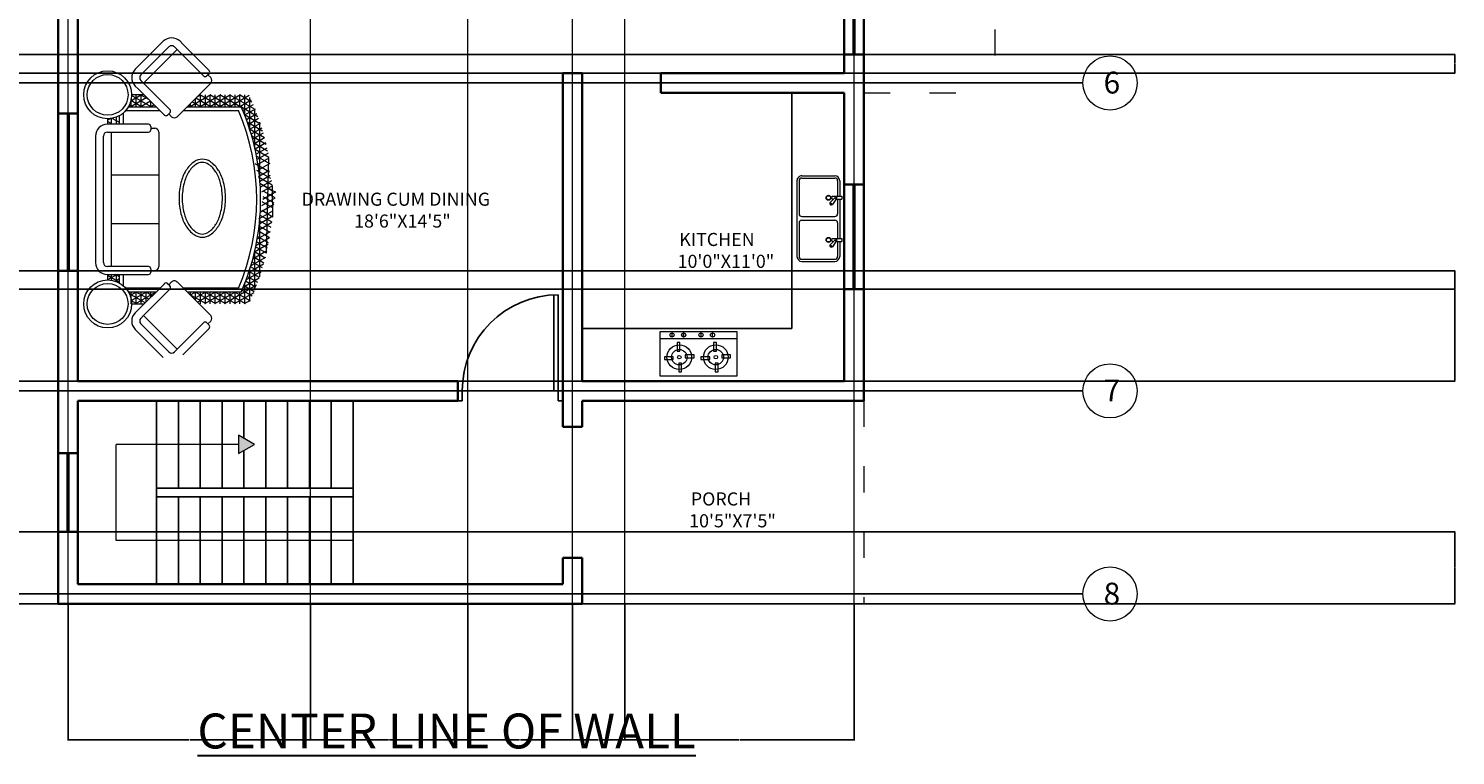
# Model space of a CAD drawing. Units: inches. Extents: x 5716 to 6907, y 12769 to 13594.
# Tile 11 of 17: x 6254 to 6907, y 12772 to 13105. Entities that reach past the tile are written whole.
import ezdxf

# ---------------------------------------------------------------- set-up
doc = ezdxf.new("R2010")
doc.units = ezdxf.units.IN
doc.linetypes.add('ACAD_ISO03W100', pattern=[30, 12, -18])
for name, color, linetype, lineweight in [('A-ANNO-DIMS', 2, 'Continuous', 18), ('A-ANNO-SYMB', 7, 'Continuous', 18), ('A-ANNO-TEXT', 7, 'Continuous', 30), ('A-AREA-IDEN', 7, 'Continuous', 18), ('A-DOOR', 4, 'Continuous', 25), ('A-EQPM', 8, 'Continuous', 18), ('A-FLOR-CASE', 7, 'Continuous', 25), ('A-FLOR-FIXT', 9, 'Continuous', 18), ('A-FLOR-OVHD', 8, 'ACAD_ISO03W100', 18), ('A-FLOR-STRS', 7, 'Continuous', 25), ('A-FURN', 8, 'Continuous', 18), ('A-GLAZ', 4, 'Continuous', 18), ('A-GRID', 8, 'Continuous', 13), ('A-GRID-IDEN', 7, 'Continuous', 18), ('A-WALL', 7, 'Continuous', 35)]:
    doc.layers.add(name, color=color, linetype=linetype, lineweight=lineweight)
doc.styles.get("Standard").update_dxf_attribs({"font": 'arial.ttf'})
doc.dimstyles.get("Standard").update_dxf_attribs({"dimtxt": 0.18, "dimasz": 0.18, "dimexe": 0.18, "dimexo": 0.0625, "dimgap": 0.09, "dimtad": 0, "dimtih": 1, "dimtoh": 1, "dimdec": 4, "dimzin": 0, "dimdsep": 46, "dimtxsty": 'Standard', "dimcen": 0.09, "dimadec": 0, "dimazin": 0, "dimtfac": 1, "dimtdec": 4, "dimtofl": 0, "dimtmove": 0, "dimatfit": 3, "dimfxl": 1, "dimtolj": 1, "dimtzin": 0, "dimarcsym": 0})

# ---------------------------------------------------------------- blocks, each defined once
blk = doc.blocks.new('A$C7A76439A')
for p, q in [((2799, 2282), (1199, 2282)), ((1199, 2182), (2799, 2182)), ((949, 1978), (1036, 2128)), ((959, 2017), (1049, 2017)), ((994, 1978), (964, 2030)), ((976, 2080), (1049, 2080)), ((1049, 2128), (980, 2128)), ((1049, 2008), (980, 2128)), ((1021, 1978), (1049, 2027)), ((1049, 2132), (1049, 2082)), ((1049, 2082), (1049, 1612)), ((1149, 1612), (1149, 2132)), ((2849, 2082), (1149, 2082)), ((1695, 2082), (1695, 1482)), ((2308, 2082), (2308, 1482)), ((2849, 2132), (2849, 1612)), ((2949, 2082), (2949, 2132)), ((3018, 2128), (2949, 2128)), ((2949, 2068), (2984, 2128)), ((2949, 1612), (2949, 2082)), ((2949, 2080), (3021, 2080)), ((2949, 2017), (3039, 2017)), ((2970, 1978), (3023, 2071)), ((3019, 2095), (3000, 2128)), ((3042, 1978), (3050, 1992)), ((677, 1830), (827, 1830)), ((677, 1758), (718, 1828)), ((677, 1825), (677, 1667)), ((690, 1655), (805, 1853)), ((827, 1642), (720, 1828)), ((827, 1767), (783, 1844)), ((827, 1517), (827, 1865)), ((877, 1467), (877, 1901)), ((905, 1928), (1049, 1928)), ((941, 1978), (1049, 1978)), ((2949, 1978), (3057, 1978)), ((2949, 1928), (3093, 1928)), ((3121, 1901), (3121, 1467)), ((3171, 1865), (3171, 1517)), ((3171, 1826), (3188, 1856)), ((3171, 1701), (3247, 1834)), ((3286, 1633), (3171, 1833)), ((3171, 1830), (3268, 1830)), ((3171, 1576), (3314, 1825)), ((3321, 1698), (3241, 1836)), ((3321, 1823), (3320, 1825)), ((3321, 1667), (3321, 1825)), ((354, 1779), (0, 1425)), ((71, 1354), (424, 1708)), ((106, 1248), (530, 1673)), ((530, 1673), (495, 1708)), ((863, 1340), (530, 1673)), ((601, 1743), (566, 1779)), ((933, 1411), (601, 1743)), ((827, 1517), (677, 1777)), ((677, 1767), (827, 1767)), ((677, 1705), (827, 1705)), ((702, 1642), (827, 1642)), ((736, 1609), (827, 1768)), ((781, 1563), (827, 1643)), ((3065, 1411), (3397, 1743)), ((3135, 1340), (3468, 1673)), ((3171, 1767), (3321, 1767)), ((3241, 1587), (3171, 1708)), ((3171, 1705), (3321, 1705)), ((3260, 1607), (3321, 1711)), ((3397, 1743), (3432, 1779)), ((3468, 1673), (3503, 1708)), ((3892, 1248), (3468, 1673)), ((3927, 1354), (3574, 1708)), ((3644, 1779), (3998, 1425)), ((765, 1580), (827, 1580)), ((1099, 1582), (1079, 1582)), ((1119, 1582), (1099, 1582)), ((1099, 1582), (1099, 1532)), ((2849, 1482), (1149, 1482)), ((2899, 1582), (2879, 1582)), ((2919, 1582), (2899, 1582)), ((2899, 1582), (2899, 1532)), ((3195, 1541), (3171, 1583)), ((3171, 1580), (3233, 1580)), ((3171, 1517), (3171, 1517)), ((106, 1248), (71, 1284)), ((905, 1340), (933, 1369)), ((919, 1354), (955, 1319)), ((3079, 1354), (3043, 1319)), ((3093, 1340), (3065, 1369)), ((3892, 1248), (3927, 1284)), ((368, 845), (35, 1178)), ((438, 916), (106, 1248)), ((530, 824), (955, 1248)), ((677, 883), (798, 1092)), ((827, 1017), (789, 1083)), ((827, 441), (827, 1121)), ((877, 474), (880, 1173)), ((3468, 824), (3043, 1248)), ((3121, 1171), (3121, 474)), ((3171, 1121), (3171, 441)), ((3171, 1076), (3187, 1105)), ((3321, 823), (3171, 1083)), ((3560, 916), (3892, 1248)), ((3630, 845), (3963, 1178)), ((3998, 1213), (3963, 1178)), ((677, 758), (827, 1018)), ((677, 955), (827, 955)), ((827, 767), (698, 991)), ((724, 1017), (827, 1017)), ((827, 892), (743, 1037)), ((786, 1080), (827, 1080)), ((3171, 1080), (3212, 1080)), ((3171, 951), (3233, 1059)), ((3171, 1017), (3274, 1017)), ((3171, 826), (3279, 1013)), ((3171, 701), (3321, 961)), ((3321, 698), (3171, 958)), ((3171, 955), (3321, 955)), ((3321, 948), (3290, 1002)), ((410, 845), (438, 874)), ((424, 859), (460, 824)), ((827, 642), (677, 902)), ((677, 633), (827, 893)), ((677, 892), (827, 892)), ((677, 830), (827, 830)), ((827, 517), (677, 777)), ((677, 508), (827, 768)), ((677, 767), (827, 767)), ((3171, 892), (3321, 892)), ((3171, 576), (3321, 836)), ((3321, 573), (3171, 833)), ((3171, 830), (3321, 830)), ((3171, 767), (3321, 767)), ((3574, 859), (3538, 824)), ((3588, 845), (3560, 874)), ((677, 705), (827, 705)), ((913, 244), (677, 652)), ((677, 383), (827, 643)), ((677, 642), (827, 642)), ((677, 580), (827, 580)), ((3134, 263), (3321, 586)), ((3171, 451), (3321, 711)), ((3321, 448), (3171, 708)), ((3171, 705), (3321, 705)), ((3171, 642), (3321, 642)), ((3311, 340), (3171, 583)), ((3171, 580), (3321, 580)), ((819, 281), (677, 527)), ((677, 517), (827, 517)), ((677, 455), (827, 455)), ((722, 324), (677, 402)), ((677, 392), (944, 392)), ((717, 326), (827, 518)), ((774, 300), (850, 431)), ((832, 276), (908, 407)), ((1004, 210), (886, 416)), ((891, 252), (966, 384)), ((950, 230), (1026, 362)), ((1093, 181), (979, 379)), ((2863, 169), (2975, 363)), ((2951, 196), (3067, 398)), ((3079, 241), (3003, 373)), ((3041, 227), (3163, 437)), ((3054, 392), (3321, 392)), ((3138, 264), (3062, 396)), ((3196, 289), (3121, 419)), ((3171, 517), (3321, 517)), ((3254, 314), (3171, 458)), ((3171, 455), (3321, 455)), ((3229, 303), (3321, 461)), ((709, 330), (1121, 330)), ((853, 267), (1349, 267)), ((1010, 209), (1086, 341)), ((1021, 205), (1744, 205)), ((1180, 156), (1070, 346)), ((1070, 188), (1147, 322)), ((1132, 170), (1209, 303)), ((1265, 133), (1159, 318)), ((1194, 152), (1271, 286)), ((1349, 114), (1245, 293)), ((1256, 135), (1334, 271)), ((1320, 120), (1398, 257)), ((1431, 97), (1330, 272)), ((1384, 106), (1463, 244)), ((1511, 83), (1412, 254)), ((1449, 94), (1528, 232)), ((1590, 71), (1494, 238)), ((1514, 82), (1595, 222)), ((1581, 72), (1662, 213)), ((1706, 50), (1607, 220)), ((1643, 60), (1723, 199)), ((1785, 38), (1688, 205)), ((1709, 49), (1790, 189)), ((1852, 43), (1749, 222)), ((1934, 26), (1833, 201)), ((2014, 12), (1916, 182)), ((2169, 45), (2089, 184)), ((2100, 34), (2198, 203)), ((2234, 57), (2155, 195)), ((2180, 47), (2280, 220)), ((2299, 71), (2220, 207)), ((2254, 205), (2977, 205)), ((2261, 63), (2363, 240)), ((2363, 85), (2284, 221)), ((2344, 81), (2449, 263)), ((2452, 77), (2371, 218)), ((2518, 88), (2438, 227)), ((2449, 77), (2547, 246)), ((2584, 100), (2504, 238)), ((2529, 90), (2629, 263)), ((2648, 113), (2569, 250)), ((2610, 105), (2712, 283)), ((2712, 128), (2633, 264)), ((2649, 267), (3145, 267)), ((2693, 124), (2798, 306)), ((2775, 144), (2697, 279)), ((2837, 161), (2760, 295)), ((2777, 145), (2885, 332)), ((2899, 179), (2822, 313)), ((2877, 330), (3289, 330)), ((2960, 199), (2883, 332)), ((3020, 220), (2943, 352)), ((1320, 120), (2529, 90)), ((1775, 39), (1857, 180)), ((1775, 39), (2169, 45)), ((1887, 35), (1966, 172)), ((1952, 23), (2032, 161)), ((2093, 0), (1997, 167)), ((2018, 11), (2098, 151)), ((2084, 1), (2165, 142))]:
    blk.add_line(p, q)
for centre, radius in [((677, 2128), 303), ((677, 2128), 258), ((3321, 2128), 303), ((3321, 2128), 258)]:
    blk.add_circle(centre, radius)
for centre, radius, start, end in [((1199, 2132), 150, 90, 180), ((1199, 2132), 50, 90, 180), ((2799, 2132), 150, 0, 90), ((2799, 2132), 50, 0, 90), ((460, 1673), 150, 45, 135), ((3538, 1673), 150, 45, 135), ((460, 1673), 50, 45, 135), ((3538, 1673), 50, 45, 135), ((1079, 1612), 30, 180, 270), ((1149, 1532), 50, 180, 270), ((1119, 1612), 30, 270, 0), ((2879, 1612), 30, 180, 270), ((2849, 1532), 50, 270, 0), ((2919, 1612), 30, 270, 0), ((106, 1319), 50, 135, 225), ((884, 1362), 30, 225, 315), ((912, 1390), 30, 315, 45), ((919, 1284), 50, 315, 45), ((3079, 1284), 50, 135, 225), ((3086, 1390), 30, 135, 225), ((3114, 1362), 30, 225, 315), ((3892, 1319), 50, 315, 45), ((3892, 1319), 150, 315, 45), ((1851, 828), 362, 120.7882, 145.1939), ((1851, 828), 322, 120.7882, 145.1939), ((1949, 662), 555, 103.8638, 120.7882), ((1949, 662), 515, 103.8638, 120.7882), ((2014, 400), 825, 90, 103.8638), ((2014, 400), 785, 90, 103.8638), ((2014, 400), 825, 76.1362, 90), ((2014, 400), 785, 76.1362, 90), ((2079, 662), 515, 59.2118, 76.1362), ((2079, 662), 555, 59.2118, 76.1362), ((2177, 828), 322, 34.8061, 59.2118), ((2177, 828), 362, 34.8061, 59.2118), ((417, 895), 30, 315, 45), ((1702, 931), 181, 145.1939, 180), ((1702, 931), 181, 180, 214.8061), ((1702, 931), 141, 145.1939, 180), ((1702, 931), 141, 180, 214.8061), ((2326, 931), 141, 0, 34.8061), ((2326, 931), 141, 325.1939, 0), ((2326, 931), 181, 0, 34.8061), ((2326, 931), 181, 325.1939, 0), ((3581, 895), 30, 135, 225), ((389, 867), 30, 225, 315), ((495, 859), 50, 225, 315), ((1851, 1035), 362, 214.8061, 239.2118), ((1851, 1035), 322, 214.8061, 239.2118), ((1949, 1200), 555, 239.2118, 256.1362), ((1949, 1200), 515, 239.2118, 256.1362), ((2079, 1200), 515, 283.8638, 300.7882), ((2079, 1200), 555, 283.8638, 300.7882), ((2177, 1035), 322, 300.7882, 325.1939), ((2177, 1035), 362, 300.7882, 325.1939), ((3503, 859), 50, 225, 315), ((3609, 867), 30, 225, 315), ((2014, 1462), 825, 256.1362, 270), ((2014, 1462), 785, 256.1362, 270), ((2014, 1462), 785, 270, 283.8638), ((2014, 1462), 825, 270, 283.8638), ((1999, 3092), 2899, 246.1589, 293.8411), ((1999, 3092), 2849, 246.8124, 293.1876)]:
    blk.add_arc(centre, radius, start, end)
blk = doc.blocks.new('A$C233D5AEA')
at = {"ltscale": 1000}
for p, q in [((20, 613), (20, 755)), ((40, 613), (40, 755)), ((375, 800), (65, 800)), ((375, 780), (65, 780)), ((400, 440), (400, 755)), ((420, 45), (420, 755)), ((55, 613), (0, 613)), ((0, 586), (0, 613)), ((89, 586), (0, 586)), ((20, 218), (20, 586)), ((40, 440), (40, 586)), ((51, 606), (87, 664)), ((112, 647), (63, 598)), ((88, 613), (78, 613)), ((87, 664), (112, 647)), ((375, 415), (65, 415)), ((40, 218), (40, 355)), ((51, 211), (87, 268)), ((375, 380), (65, 380)), ((87, 268), (112, 252)), ((400, 45), (400, 355)), ((55, 218), (0, 218)), ((0, 191), (0, 218)), ((89, 191), (0, 191)), ((20, 45), (20, 191)), ((40, 45), (40, 191)), ((112, 252), (63, 202)), ((88, 218), (78, 218)), ((375, 20), (65, 20)), ((375, 0), (65, 0))]:
    blk.add_line(p, q, dxfattribs=at)
for centre, radius in [((55, 600), 7.79), ((125, 599), 23.1), ((125, 599), 19.5), ((55, 204), 7.79), ((125, 205), 23.1), ((125, 205), 19.5)]:
    blk.add_circle(centre, radius, dxfattribs=at)
for centre, radius, start, end in [((65, 755), 45, 90, 180), ((65, 755), 25, 90, 180), ((375, 755), 45, 0, 90), ((375, 755), 25, 0, 90), ((98, 652), 15.3, 340.4622, 131.655), ((82, 599), 14.9, 296.6237, 67.0796), ((65, 440), 25, 180, 270), ((375, 440), 25, 270, 0), ((65, 355), 25, 90, 180), ((98, 257), 15.3, 340.4691, 131.6481), ((375, 355), 25, 0, 90), ((82, 204), 14.9, 296.6237, 67.0796), ((65, 45), 45, 180, 270), ((65, 45), 25, 180, 270), ((375, 45), 45, 270, 0), ((375, 45), 25, 270, 0)]:
    blk.add_arc(centre, radius, start, end, dxfattribs=at)
blk = doc.blocks.new('A$C3BE07067')
at = {"rotation": 270}
blk.add_blockref('A$C233D5AEA', (0, 420), dxfattribs=at)
blk = doc.blocks.new('A$C67D72025')
at = {"ltscale": 1000}
for p, q in [((386, 234), (386, 209)), ((465, 234), (386, 234)), ((386, 209), (465, 209)), ((465, 209), (465, 234)), ((694, 60), (0, 60))]:
    blk.add_line(p, q, dxfattribs=at)
for points in [[(694, 397), (0, 397), (0, 0), (694, 0)], [(196, 284), (196, 362), (171, 362), (171, 284)], [(523, 284), (523, 362), (499, 362), (499, 284)], [(137, 234), (58, 234), (58, 209), (137, 209)], [(186, 175), (186, 96), (211, 96), (211, 175)], [(245, 225), (324, 225), (324, 250), (245, 250)], [(514, 175), (514, 96), (539, 96), (539, 175)], [(573, 225), (652, 225), (652, 250), (573, 250)], [(223, 47), (220, 47), (220, 10), (223, 10)], [(326, 47), (322, 47), (322, 10), (326, 10)], [(483, 47), (479, 47), (479, 10), (483, 10)], [(585, 47), (582, 47), (582, 10), (585, 10)]]:
    blk.add_lwpolyline(points, close=True, dxfattribs=at)
for centre, radius in [((191, 229), 111), ((191, 229), 69.6), ((519, 229), 111), ((519, 229), 69.6), ((191, 229), 15.5), ((519, 229), 15.5), ((220, 29), 18.6), ((324, 29), 18.6), ((480, 29), 18.6), ((584, 29), 18.6)]:
    blk.add_circle(centre, radius, dxfattribs=at)
blk = doc.blocks.new('DOOR-SWING-48IN')
for p, q in [((-2, 43.95), (-2, 0)), ((0, 44), (0, 0)), ((-46, 0), (-44, 0)), ((-44, -4.5), (-46, -4.5)), ((-44, 0), (-44, -4.5)), ((0, 0), (-2, 0)), ((2, 0), (0, 0)), ((0, 0), (0, -4.5)), ((0, -4.5), (2, -4.5))]:
    blk.add_line(p, q)
blk.add_arc((0, 0), 44, 90, 180)
blk = doc.blocks.new('WIN-GLAZING-72IN')
for p, q in [((0, 0), (0, -72)), ((1, 0), (1, -72))]:
    blk.add_line(p, q)
blk = doc.blocks.new('WIN-GLAZING-48IN')
for p, q in [((0, 0), (0, 48)), ((1, 0), (1, 48))]:
    blk.add_line(p, q)
blk = doc.blocks.new('WIN-GLAZING-36IN')
for p, q in [((0, 0), (0, 36)), ((1, 0), (1, 36))]:
    blk.add_line(p, q)
blk = doc.blocks.new('STAIR-RETURN-FLIGHT')
for p, q in [((0, 84), (0, 44)), ((10, 84), (10, 44)), ((20, 84), (20, 44)), ((30, 84), (30, 44)), ((40, 84), (40, 66.79)), ((50, 84), (50, 44)), ((60, 84), (60, 44)), ((70, 84), (70, 44)), ((80, 84), (80, 44)), ((90, 84), (90, 44)), ((40, 61.21), (40, 44)), ((0, 44), (90, 44)), ((0, 40), (0, 44)), ((0, 40), (90, 40)), ((0, 40), (0, 0)), ((10, 40), (10, 0)), ((20, 40), (20, 0)), ((30, 40), (30, 0)), ((40, 40), (40, 0)), ((50, 40), (50, 0)), ((60, 40), (60, 0)), ((70, 40), (70, 0)), ((80, 40), (80, 0)), ((90, 40), (90, 44)), ((90, 40), (90, 0))]:
    blk.add_line(p, q)
blk = doc.blocks.new('COUNTER-L-KITCHEN')
for p in [(0, 108), (-96, 0)]:
    blk.add_line(p, (0, 0))
blk = doc.blocks.new('*D52')
at = {"layer": 'A-ANNO-DIMS', "color": 0, "lineweight": -2, "transparency": 16777216}
for p, q in [((6267.34, 13440.15), (5716.04, 13440.15)), ((5716.22, 13439.97), (5716.22, 13140.83)), ((5716.22, 12841.33), (5716.22, 13140.47)), ((6267.34, 12841.15), (5716.04, 12841.15))]:
    blk.add_line(p, q, dxfattribs=at)
at = {"layer": 'A-ANNO-DIMS', "color": 0, "transparency": 16777216}
for points in [[(5716.19, 13439.97), (5716.25, 13439.97), (5716.22, 13440.15)], [(5716.19, 12841.33), (5716.25, 12841.33), (5716.22, 12841.15)]]:
    blk.add_solid(points, dxfattribs=at)
at = {"layer": 'Defpoints', "color": 0, "transparency": 16777216}
for p in [(6267.41, 13440.15), (5716.22, 12841.15), (6267.41, 12841.15)]:
    blk.add_point(p, dxfattribs=at)
at = {"layer": 'A-ANNO-DIMS', "color": 0, "transparency": 16777216, "insert": (5716.22, 13140.65), "char_height": 0.18, "attachment_point": 5}
blk.add_mtext('\\A1;599', dxfattribs=at)
blk = doc.blocks.new('*D53')
at = {"layer": 'A-ANNO-DIMS', "color": 0, "lineweight": -2, "transparency": 16777216}
for p, q in [((6271.91, 12841.09), (6271.91, 12778.62)), ((6382.91, 12841.09), (6382.91, 12778.62)), ((6272.09, 12778.8), (6327.14, 12778.8)), ((6382.73, 12778.8), (6327.67, 12778.8))]:
    blk.add_line(p, q, dxfattribs=at)
at = {"layer": 'A-ANNO-DIMS', "color": 0, "transparency": 16777216}
for points in [[(6272.09, 12778.83), (6272.09, 12778.77), (6271.91, 12778.8)], [(6382.73, 12778.83), (6382.73, 12778.77), (6382.91, 12778.8)]]:
    blk.add_solid(points, dxfattribs=at)
at = {"layer": 'Defpoints', "color": 0, "transparency": 16777216}
for p in [(6271.91, 12841.15), (6382.91, 12841.15), (6382.91, 12778.8)]:
    blk.add_point(p, dxfattribs=at)
at = {"layer": 'A-ANNO-DIMS', "color": 0, "transparency": 16777216, "insert": (6327.41, 12778.8), "char_height": 0.18, "attachment_point": 5}
blk.add_mtext('\\A1;111', dxfattribs=at)
blk = doc.blocks.new('*D54')
at = {"layer": 'A-ANNO-DIMS', "color": 0, "lineweight": -2, "transparency": 16777216}
for p, q in [((6382.91, 12841.09), (6382.91, 12778.62)), ((6454.91, 12841.09), (6454.91, 12778.62)), ((6383.09, 12778.8), (6418.69, 12778.8)), ((6454.73, 12778.8), (6419.12, 12778.8))]:
    blk.add_line(p, q, dxfattribs=at)
at = {"layer": 'A-ANNO-DIMS', "color": 0, "transparency": 16777216}
for points in [[(6383.09, 12778.83), (6383.09, 12778.77), (6382.91, 12778.8)], [(6454.73, 12778.83), (6454.73, 12778.77), (6454.91, 12778.8)]]:
    blk.add_solid(points, dxfattribs=at)
at = {"layer": 'Defpoints', "color": 0, "transparency": 16777216}
for p in [(6382.91, 12841.15), (6454.91, 12841.15), (6454.91, 12778.8)]:
    blk.add_point(p, dxfattribs=at)
at = {"layer": 'A-ANNO-DIMS', "color": 0, "transparency": 16777216, "insert": (6418.91, 12778.8), "char_height": 0.18, "attachment_point": 5}
blk.add_mtext('\\A1;72', dxfattribs=at)
blk = doc.blocks.new('*D55')
at = {"layer": 'A-ANNO-DIMS', "color": 0, "lineweight": -2, "transparency": 16777216}
for p, q in [((6454.91, 12841.09), (6454.91, 12778.62)), ((6502.91, 12841.09), (6502.91, 12778.62)), ((6455.09, 12778.8), (6478.68, 12778.8)), ((6502.73, 12778.8), (6479.13, 12778.8))]:
    blk.add_line(p, q, dxfattribs=at)
at = {"layer": 'A-ANNO-DIMS', "color": 0, "transparency": 16777216}
for points in [[(6455.09, 12778.83), (6455.09, 12778.77), (6454.91, 12778.8)], [(6502.73, 12778.83), (6502.73, 12778.77), (6502.91, 12778.8)]]:
    blk.add_solid(points, dxfattribs=at)
at = {"layer": 'Defpoints', "color": 0, "transparency": 16777216}
for p in [(6454.91, 12841.15), (6502.91, 12841.15), (6502.91, 12778.8)]:
    blk.add_point(p, dxfattribs=at)
at = {"layer": 'A-ANNO-DIMS', "color": 0, "transparency": 16777216, "insert": (6478.91, 12778.8), "char_height": 0.18, "attachment_point": 5}
blk.add_mtext('\\A1;48', dxfattribs=at)
blk = doc.blocks.new('*D56')
at = {"layer": 'A-ANNO-DIMS', "color": 0, "lineweight": -2, "transparency": 16777216}
for p, q in [((6502.91, 12841.09), (6502.91, 12778.62)), ((6526.91, 12841.09), (6526.91, 12778.62)), ((6503.09, 12778.8), (6514.69, 12778.8)), ((6526.73, 12778.8), (6515.13, 12778.8))]:
    blk.add_line(p, q, dxfattribs=at)
at = {"layer": 'A-ANNO-DIMS', "color": 0, "transparency": 16777216}
for points in [[(6503.09, 12778.83), (6503.09, 12778.77), (6502.91, 12778.8)], [(6526.73, 12778.83), (6526.73, 12778.77), (6526.91, 12778.8)]]:
    blk.add_solid(points, dxfattribs=at)
at = {"layer": 'Defpoints', "color": 0, "transparency": 16777216}
for p in [(6502.91, 12841.15), (6526.91, 12841.15), (6526.91, 12778.8)]:
    blk.add_point(p, dxfattribs=at)
at = {"layer": 'A-ANNO-DIMS', "color": 0, "transparency": 16777216, "insert": (6514.91, 12778.8), "char_height": 0.18, "attachment_point": 5}
blk.add_mtext('\\A1;24', dxfattribs=at)
blk = doc.blocks.new('*D57')
at = {"layer": 'A-ANNO-DIMS', "color": 0, "lineweight": -2, "transparency": 16777216}
for p, q in [((6526.91, 12841.09), (6526.91, 12778.62)), ((6631.91, 12841.09), (6631.91, 12778.62)), ((6527.09, 12778.8), (6579.13, 12778.8)), ((6631.73, 12778.8), (6579.69, 12778.8))]:
    blk.add_line(p, q, dxfattribs=at)
at = {"layer": 'A-ANNO-DIMS', "color": 0, "transparency": 16777216}
for points in [[(6527.09, 12778.83), (6527.09, 12778.77), (6526.91, 12778.8)], [(6631.73, 12778.83), (6631.73, 12778.77), (6631.91, 12778.8)]]:
    blk.add_solid(points, dxfattribs=at)
at = {"layer": 'Defpoints', "color": 0, "transparency": 16777216}
for p in [(6526.91, 12841.15), (6631.91, 12841.15), (6631.91, 12778.8)]:
    blk.add_point(p, dxfattribs=at)
at = {"layer": 'A-ANNO-DIMS', "color": 0, "transparency": 16777216, "insert": (6579.41, 12778.8), "char_height": 0.18, "attachment_point": 5}
blk.add_mtext('\\A1;105', dxfattribs=at)
blk = doc.blocks.new('*D62')
at = {"layer": 'A-ANNO-DIMS', "color": 0, "lineweight": -2, "transparency": 16777216}
for p, q in [((6736.67, 13120.65), (5716.04, 13120.65)), ((5716.22, 13120.47), (5716.22, 13100.33)), ((5716.22, 13079.83), (5716.22, 13099.97)), ((6736.67, 13079.65), (5716.04, 13079.65))]:
    blk.add_line(p, q, dxfattribs=at)
at = {"layer": 'A-ANNO-DIMS', "color": 0, "transparency": 16777216}
for points in [[(5716.19, 13120.47), (5716.25, 13120.47), (5716.22, 13120.65)], [(5716.19, 13079.83), (5716.25, 13079.83), (5716.22, 13079.65)]]:
    blk.add_solid(points, dxfattribs=at)
at = {"layer": 'Defpoints', "color": 0, "transparency": 16777216}
for p in [(6736.73, 13120.65), (5716.22, 13079.65), (6736.73, 13079.65)]:
    blk.add_point(p, dxfattribs=at)
at = {"layer": 'A-ANNO-DIMS', "color": 0, "transparency": 16777216, "insert": (5716.22, 13100.15), "char_height": 0.18, "attachment_point": 5}
blk.add_mtext('\\A1;41', dxfattribs=at)
blk = doc.blocks.new('*D63')
at = {"layer": 'A-ANNO-DIMS', "color": 0, "lineweight": -2, "transparency": 16777216}
for p, q in [((6736.67, 13079.65), (5716.04, 13079.65)), ((5716.22, 13079.47), (5716.22, 13009.33)), ((5716.22, 12938.83), (5716.22, 13008.97)), ((6736.67, 12938.65), (5716.04, 12938.65))]:
    blk.add_line(p, q, dxfattribs=at)
at = {"layer": 'A-ANNO-DIMS', "color": 0, "transparency": 16777216}
for points in [[(5716.19, 13079.47), (5716.25, 13079.47), (5716.22, 13079.65)], [(5716.19, 12938.83), (5716.25, 12938.83), (5716.22, 12938.65)]]:
    blk.add_solid(points, dxfattribs=at)
at = {"layer": 'Defpoints', "color": 0, "transparency": 16777216}
for p in [(6736.73, 13079.65), (5716.22, 12938.65), (6736.73, 12938.65)]:
    blk.add_point(p, dxfattribs=at)
at = {"layer": 'A-ANNO-DIMS', "color": 0, "transparency": 16777216, "insert": (5716.22, 13009.15), "char_height": 0.18, "attachment_point": 5}
blk.add_mtext('\\A1;141', dxfattribs=at)
blk = doc.blocks.new('*D64')
at = {"layer": 'A-ANNO-DIMS', "color": 0, "lineweight": -2, "transparency": 16777216}
for p, q in [((6736.67, 12938.65), (5716.04, 12938.65)), ((5716.22, 12938.47), (5716.22, 12892.33)), ((5716.22, 12845.83), (5716.22, 12891.97)), ((6736.67, 12845.65), (5716.04, 12845.65))]:
    blk.add_line(p, q, dxfattribs=at)
at = {"layer": 'A-ANNO-DIMS', "color": 0, "transparency": 16777216}
for points in [[(5716.19, 12938.47), (5716.25, 12938.47), (5716.22, 12938.65)], [(5716.19, 12845.83), (5716.25, 12845.83), (5716.22, 12845.65)]]:
    blk.add_solid(points, dxfattribs=at)
at = {"layer": 'Defpoints', "color": 0, "transparency": 16777216}
for p in [(6736.73, 12938.65), (5716.22, 12845.65), (6736.73, 12845.65)]:
    blk.add_point(p, dxfattribs=at)
at = {"layer": 'A-ANNO-DIMS', "color": 0, "transparency": 16777216, "insert": (5716.22, 12892.15), "char_height": 0.18, "attachment_point": 5}
blk.add_mtext('\\A1;93', dxfattribs=at)
blk = doc.blocks.new('*D67')
at = {"layer": 'A-ANNO-DIMS', "color": 0, "lineweight": -2, "transparency": 16777216}
for p, q in [((5819.09, 12874.15), (6907.26, 12874.15)), ((6907.08, 12873.97), (6907.08, 12857.83)), ((6907.08, 12841.33), (6907.08, 12857.47)), ((5819.09, 12841.15), (6907.26, 12841.15))]:
    blk.add_line(p, q, dxfattribs=at)
at = {"layer": 'A-ANNO-DIMS', "color": 0, "transparency": 16777216}
for points in [[(6907.05, 12873.97), (6907.11, 12873.97), (6907.08, 12874.15)], [(6907.05, 12841.33), (6907.11, 12841.33), (6907.08, 12841.15)]]:
    blk.add_solid(points, dxfattribs=at)
at = {"layer": 'Defpoints', "color": 0, "transparency": 16777216}
for p in [(5819.02, 12874.15), (6907.08, 12874.15), (5819.02, 12841.15)]:
    blk.add_point(p, dxfattribs=at)
at = {"layer": 'A-ANNO-DIMS', "color": 0, "transparency": 16777216, "insert": (6907.08, 12857.65), "char_height": 0.18, "attachment_point": 5}
blk.add_mtext('\\A1;33', dxfattribs=at)
blk = doc.blocks.new('*D68')
at = {"layer": 'A-ANNO-DIMS', "color": 0, "lineweight": -2, "transparency": 16777216}
for p, q in [((5828.09, 12993.65), (6907.26, 12993.65)), ((6907.08, 12993.47), (6907.08, 12968.58)), ((6907.08, 12943.33), (6907.08, 12968.22)), ((5828.09, 12943.15), (6907.26, 12943.15))]:
    blk.add_line(p, q, dxfattribs=at)
at = {"layer": 'A-ANNO-DIMS', "color": 0, "transparency": 16777216}
for points in [[(6907.05, 12993.47), (6907.11, 12993.47), (6907.08, 12993.65)], [(6907.05, 12943.33), (6907.11, 12943.33), (6907.08, 12943.15)]]:
    blk.add_solid(points, dxfattribs=at)
at = {"layer": 'Defpoints', "color": 0, "transparency": 16777216}
for p in [(5828.02, 12993.65), (6907.08, 12993.65), (5828.02, 12943.15)]:
    blk.add_point(p, dxfattribs=at)
at = {"layer": 'A-ANNO-DIMS', "color": 0, "transparency": 16777216, "insert": (6907.08, 12968.4), "char_height": 0.18, "attachment_point": 5}
blk.add_mtext('\\A1;50.5', dxfattribs=at)
blk = doc.blocks.new('*D72')
at = {"layer": 'A-ANNO-DIMS', "color": 0, "lineweight": -2, "transparency": 16777216}
for p, q in [((6188.09, 12985.15), (6907.26, 12985.15)), ((6907.08, 12984.97), (6907.08, 12964.33)), ((6907.08, 12943.33), (6907.08, 12963.97)), ((6179.09, 12943.15), (6907.26, 12943.15))]:
    blk.add_line(p, q, dxfattribs=at)
at = {"layer": 'A-ANNO-DIMS', "color": 0, "transparency": 16777216}
for points in [[(6907.05, 12984.97), (6907.11, 12984.97), (6907.08, 12985.15)], [(6907.05, 12943.33), (6907.11, 12943.33), (6907.08, 12943.15)]]:
    blk.add_solid(points, dxfattribs=at)
at = {"layer": 'Defpoints', "color": 0, "transparency": 16777216}
for p in [(6188.02, 12985.15), (6907.08, 12985.15), (6179.02, 12943.15)]:
    blk.add_point(p, dxfattribs=at)
at = {"layer": 'A-ANNO-DIMS', "color": 0, "transparency": 16777216, "insert": (6907.08, 12964.15), "char_height": 0.18, "attachment_point": 5}
blk.add_mtext('\\A1;42', dxfattribs=at)
blk = doc.blocks.new('*D73')
at = {"layer": 'A-ANNO-DIMS', "color": 0, "lineweight": -2, "transparency": 16777216}
for p, q in [((6188.09, 13092.65), (6907.26, 13092.65)), ((6907.08, 13092.47), (6907.08, 13088.58)), ((6907.08, 13084.33), (6907.08, 13088.22)), ((6179.09, 13084.15), (6907.26, 13084.15))]:
    blk.add_line(p, q, dxfattribs=at)
at = {"layer": 'A-ANNO-DIMS', "color": 0, "transparency": 16777216}
for points in [[(6907.05, 13092.47), (6907.11, 13092.47), (6907.08, 13092.65)], [(6907.05, 13084.33), (6907.11, 13084.33), (6907.08, 13084.15)]]:
    blk.add_solid(points, dxfattribs=at)
at = {"layer": 'Defpoints', "color": 0, "transparency": 16777216}
for p in [(6188.02, 13092.65), (6907.08, 13092.65), (6179.02, 13084.15)]:
    blk.add_point(p, dxfattribs=at)
at = {"layer": 'A-ANNO-DIMS', "color": 0, "transparency": 16777216, "insert": (6907.08, 13088.4), "char_height": 0.18, "attachment_point": 5}
blk.add_mtext('\\A1;8.5', dxfattribs=at)

msp = doc.modelspace()

# ---------------------------------------------------------------- hatches: boundary and pattern name
at = {"layer": 'A-ANNO-SYMB'}
h = msp.add_hatch(color=256, dxfattribs=at)
h.dxf.hatch_style = 1
h.paths.add_polyline_path([(6357.24, 12914.15), (6349.99, 12918.34), (6349.99, 12909.96)])

# ---------------------------------------------------------------- linework, layer by layer
for p, q in [((6293.86, 12870.15), (6293.86, 12914.15)), ((6349.99, 12914.15), (6293.86, 12914.15)), ((6402.41, 12870.15), (6293.86, 12870.15))]:
    msp.add_line(p, q, dxfattribs=at)
msp.add_lwpolyline([(6357.24, 12914.15), (6349.99, 12918.34), (6349.99, 12909.96)], close=True, dxfattribs=at)
at = {"layer": 'A-FLOR-OVHD'}
for p, q in [((6696.41, 13194.15), (6696.41, 13075.15)), ((6636.41, 13075.15), (6696.41, 13075.15)), ((6636.41, 12934.15), (6636.41, 12841.15)), ((6507.41, 12841.15), (6636.41, 12841.15))]:
    msp.add_line(p, q, dxfattribs=at)
at = {"layer": 'A-GRID'}
for p, q in [((6271.91, 12841.15), (6271.91, 13514.96)), ((6382.91, 12841.15), (6382.91, 13514.96)), ((6454.91, 12841.15), (6454.91, 13514.96)), ((6502.91, 12841.15), (6502.91, 13514.96)), ((6526.91, 12841.15), (6526.91, 13514.96)), ((6631.91, 12841.15), (6631.91, 13514.96)), ((6267.41, 13079.65), (6736.73, 13079.65)), ((6267.41, 12938.65), (6736.73, 12938.65)), ((6267.41, 12845.65), (6736.73, 12845.65))]:
    msp.add_line(p, q, dxfattribs=at)
at = {"layer": 'A-GRID-IDEN'}
for centre in [(6749.12, 13079.65), (6749.12, 12938.65), (6749.12, 12845.65)]:
    msp.add_circle(centre, 12.4, dxfattribs=at)
at = {"layer": 'A-WALL'}
for p, q in [((6267.41, 13440.15), (6267.41, 12841.15)), ((6627.41, 13149.15), (6627.41, 13084.15)), ((6636.41, 13149.15), (6636.41, 12934.15)), ((6276.41, 13116.15), (6276.41, 12943.15)), ((6627.41, 13092.65), (6636.41, 13092.65)), ((6498.41, 13084.15), (6498.41, 12922.15)), ((6498.41, 13084.15), (6507.41, 13084.15)), ((6507.41, 13084.15), (6507.41, 12943.15)), ((6543.41, 13084.15), (6543.41, 13075.15)), ((6543.41, 13084.15), (6627.41, 13084.15)), ((6543.41, 13075.15), (6627.41, 13075.15)), ((6627.41, 13075.15), (6627.41, 12943.15)), ((6276.41, 13065.65), (6267.41, 13065.65)), ((6627.41, 13033.15), (6636.41, 13033.15)), ((6276.41, 12993.65), (6267.41, 12993.65)), ((6627.41, 12985.15), (6636.41, 12985.15)), ((6276.41, 12943.15), (6450.41, 12943.15)), ((6450.41, 12943.15), (6450.41, 12934.15)), ((6507.41, 12943.15), (6627.41, 12943.15)), ((6276.41, 12934.15), (6276.41, 12850.15)), ((6276.41, 12934.15), (6450.41, 12934.15)), ((6507.41, 12934.15), (6507.41, 12922.15)), ((6507.41, 12934.15), (6636.41, 12934.15)), ((6498.41, 12922.15), (6507.41, 12922.15)), ((6276.41, 12910.15), (6267.41, 12910.15)), ((6276.41, 12874.15), (6267.41, 12874.15)), ((6498.41, 12862.15), (6498.41, 12850.15)), ((6498.41, 12862.15), (6507.41, 12862.15)), ((6507.41, 12862.15), (6507.41, 12841.15)), ((6276.41, 12850.15), (6498.41, 12850.15)), ((6267.41, 12841.15), (6507.41, 12841.15))]:
    msp.add_line(p, q, dxfattribs=at)

# ---------------------------------------------------------------- block references
at = {"layer": 'A-DOOR'}
msp.add_blockref('DOOR-SWING-48IN', (6496.41, 12938.65), dxfattribs=at)
at = {"layer": 'A-EQPM', "xscale": 0.0509457092912183, "yscale": 0.0509457092912183, "zscale": 0.0509457092912183, "rotation": 180}
msp.add_blockref('A$C67D72025', (6578.27, 12965.75), dxfattribs=at)
at = {"layer": 'A-FLOR-CASE'}
msp.add_blockref('COUNTER-L-KITCHEN', (6603.41, 12967.15), dxfattribs=at)
at = {"layer": 'A-FLOR-FIXT', "xscale": 0.0489344977334652, "yscale": 0.0489344977334652, "zscale": 0.0489344977334652, "rotation": 270}
msp.add_blockref('A$C3BE07067', (6605.72, 13037.09), dxfattribs=at)
at = {"layer": 'A-FLOR-STRS'}
msp.add_blockref('STAIR-RETURN-FLIGHT', (6312.41, 12850.15), dxfattribs=at)
at = {"layer": 'A-FURN', "xscale": 0.0362164969968974, "yscale": 0.0362164969968974, "zscale": 0.0362164969968974, "rotation": 90}
msp.add_blockref('A$C7A76439A', (6367.07, 12953.94), dxfattribs=at)
at = {"layer": 'A-GLAZ'}
for name, p in [('WIN-GLAZING-48IN', (6631.41, 13092.65)), ('WIN-GLAZING-72IN', (6271.41, 13065.65)), ('WIN-GLAZING-48IN', (6631.41, 12985.15)), ('WIN-GLAZING-36IN', (6271.41, 12874.15))]:
    msp.add_blockref(name, p, dxfattribs=at)

# ---------------------------------------------------------------- texts
at = {"layer": 'A-ANNO-TEXT', "insert": (6331.1, 12790.92), "char_height": 16, "attachment_point": 1}
msp.add_mtext_dynamic_manual_height_columns('{\\LCENTER LINE OF WALL}', width=852.8728, gutter_width=12.5, heights=[0], dxfattribs=at)
at = {"layer": 'A-AREA-IDEN', "attachment_point": 1}
for s, width, heights, insert, char_height in [('DRAWING CUM DINING\\P^I18\'6"X14\'5"', 158.347, [0], (6378.87, 13029.41), 6), (' {\\H2.4x;KITCHEN\\P10\'0"X11\'0"}', 81.2135, [0], (6551.05, 13010.98), 2.5), (' {\\H2.4x;PORCH\\P10\'5"X7\'5"}', 95.0073, [19.73], (6556.34, 12892.17), 2.5)]:
    msp.add_mtext_dynamic_manual_height_columns(s, width=width, gutter_width=12.5, heights=heights, dxfattribs=dict(at, insert=insert, char_height=char_height))
at = {"layer": 'A-GRID-IDEN', "char_height": 10, "attachment_point": 1}
for s, insert in [('6', (6746.18, 13084.81)), ('7', (6746.18, 12943.81)), ('8', (6746.18, 12850.81))]:
    msp.add_mtext_dynamic_manual_height_columns(s, width=121.9272, gutter_width=12.5, heights=[0], dxfattribs=dict(at, insert=insert))

# ---------------------------------------------------------------- dimensions: what is measured, and where the dimension line sits
at = {"layer": 'A-ANNO-DIMS'}
for base, p1, p2, override, picture, middle in [((5716.22, 12841.15), (6267.41, 13440.15), (6267.41, 12841.15), {"dimdec": 0, "dimlfac": 1, "dimrnd": 0, "dimzin": 0, "dimdsep": 46, "dimlunit": 2}, '*D52', (5716.22, 13140.65)), ((5716.22, 13079.65), (6736.73, 13120.65), (6736.73, 13079.65), {"dimdec": 0, "dimlfac": 1, "dimrnd": 0, "dimzin": 0, "dimdsep": 46, "dimlunit": 2}, '*D62', (5716.22, 13100.15)), ((6907.08, 13092.65), (6179.02, 13084.15), (6188.02, 13092.65), {"dimdec": 1, "dimlfac": 1, "dimrnd": 0, "dimzin": 0, "dimdsep": 46, "dimlunit": 2}, '*D73', (6907.08, 13088.4)), ((5716.22, 12938.65), (6736.73, 13079.65), (6736.73, 12938.65), {"dimdec": 0, "dimlfac": 1, "dimrnd": 0, "dimzin": 0, "dimdsep": 46, "dimlunit": 2}, '*D63', (5716.22, 13009.15)), ((6907.08, 12993.65), (5828.02, 12943.15), (5828.02, 12993.65), {"dimdec": 1, "dimlfac": 1, "dimrnd": 0, "dimzin": 0, "dimdsep": 46, "dimlunit": 2}, '*D68', (6907.08, 12968.4)), ((6907.08, 12985.15), (6179.02, 12943.15), (6188.02, 12985.15), {"dimdec": 0, "dimlfac": 1, "dimrnd": 0, "dimzin": 0, "dimdsep": 46, "dimlunit": 2}, '*D72', (6907.08, 12964.15)), ((5716.22, 12845.65), (6736.73, 12938.65), (6736.73, 12845.65), {"dimdec": 0, "dimlfac": 1, "dimrnd": 0, "dimzin": 0, "dimdsep": 46, "dimlunit": 2}, '*D64', (5716.22, 12892.15)), ((6907.08, 12874.15), (5819.02, 12841.15), (5819.02, 12874.15), {"dimdec": 0, "dimlfac": 1, "dimrnd": 0, "dimzin": 0, "dimdsep": 46, "dimlunit": 2}, '*D67', (6907.08, 12857.65))]:
    dim = msp.add_linear_dim(base=base, p1=p1, p2=p2, angle=90, dimstyle='Standard', override=override, dxfattribs=at)
    dim.commit()
    dim.dimension.update_dxf_attribs({"geometry": picture, "text_midpoint": middle})
for base, p1, p2, picture, middle in [((6382.91, 12778.8), (6271.91, 12841.15), (6382.91, 12841.15), '*D53', (6327.41, 12778.8)), ((6454.91, 12778.8), (6382.91, 12841.15), (6454.91, 12841.15), '*D54', (6418.91, 12778.8)), ((6502.91, 12778.8), (6454.91, 12841.15), (6502.91, 12841.15), '*D55', (6478.91, 12778.8)), ((6526.91, 12778.8), (6502.91, 12841.15), (6526.91, 12841.15), '*D56', (6514.91, 12778.8)), ((6631.91, 12778.8), (6526.91, 12841.15), (6631.91, 12841.15), '*D57', (6579.41, 12778.8))]:
    dim = msp.add_linear_dim(base=base, p1=p1, p2=p2, dimstyle='Standard', override={"dimdec": 0, "dimlfac": 1, "dimrnd": 0, "dimzin": 0, "dimdsep": 46, "dimlunit": 2}, dxfattribs=at)
    dim.commit()
    dim.dimension.update_dxf_attribs({"geometry": picture, "text_midpoint": middle})

doc.saveas('drawing.dxf')
